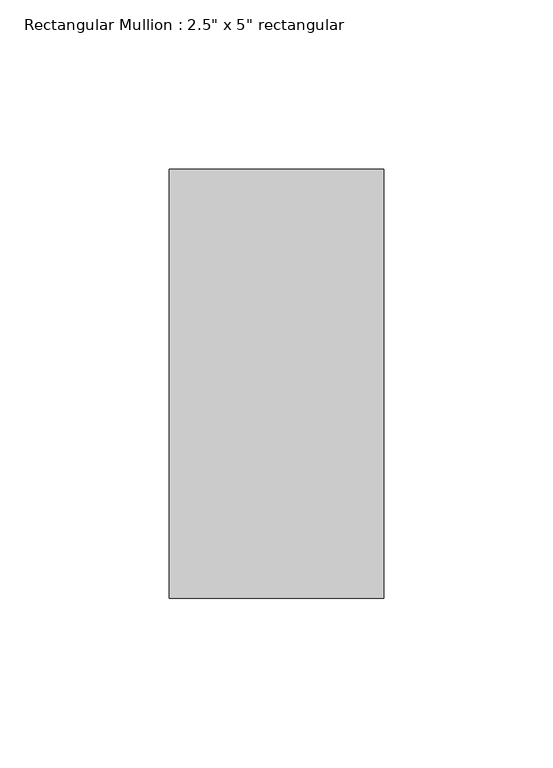
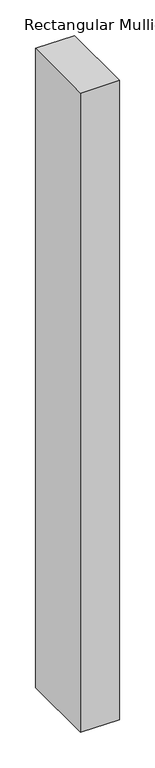
"""IFC4 building model written with IfcOpenShell, lengths in millimetres: member geometry."""

from ifc_helpers import new_model, si_unit, frame, origin, place, context, project, spatial, polyline, outline, extrude, source, transform, mapped, element, save


def member_69c8e218(model_context):
    return source(origin(), model_context, "Body", "SweptSolid", [
        extrude(outline(polyline([(0.0, 63.5), (0.0, -63.5), (-63.5, -63.5), (-63.5, 63.5), (0.0, 63.5)])), frame((0.0, 0.0, -1098.55), z_axis=(0.0, 0.0, 1.0), x_axis=(1.0, 0.0, 0.0)), (0.0, 0.0, 1.0), 1098.55),
    ])


if __name__ == "__main__":
    model = new_model("IFC4")
    model_context = context("Model", 3, world=origin())
    ifc_project = project(units=[si_unit("LENGTHUNIT", "METRE", prefix="MILLI")], contexts=[model_context])
    site = spatial("IfcSite", under=ifc_project)
    building = spatial("IfcBuilding", under=site)
    placement = place(None, origin())
    member_shape = member_69c8e218(model_context)
    element("IfcMember", 1, ObjectType="Rectangular Mullion : 2.5\" x 5\" rectangular", at=placement, inside=building, context=model_context, shape_type="MappedRepresentation", body=[
        mapped(member_shape, transform((0.0, 0.0, 0.0), x_axis=(1.0, 0.0, 0.0), y_axis=(0.0, 1.0, 0.0), z_axis=(0.0, 0.0, 1.0))),
    ])
    save(model, "model.ifc")

# Revit data of these elements
# Type "Rectangular Mullion : 2.5\" x 5\" rectangular"
#   built-in parameter 1007304 = 0.416667 (stored number, unit not read)
#   built-in parameter 1007301 = 0.104167 (stored number, unit not read)
#   built-in parameter 1007300 = 0.104167 (stored number, unit not read)
# Element 1 (IfcMember, "Rectangular Mullion : 2.5\" x 5\" rectangular")
#   Materials on its faces: "Aluminum"
# Materials
#   "Aluminum": class "Metal", colour RGB 247 247 247, transparency 0, Description = "Aluminum 6061", Cost = 0
